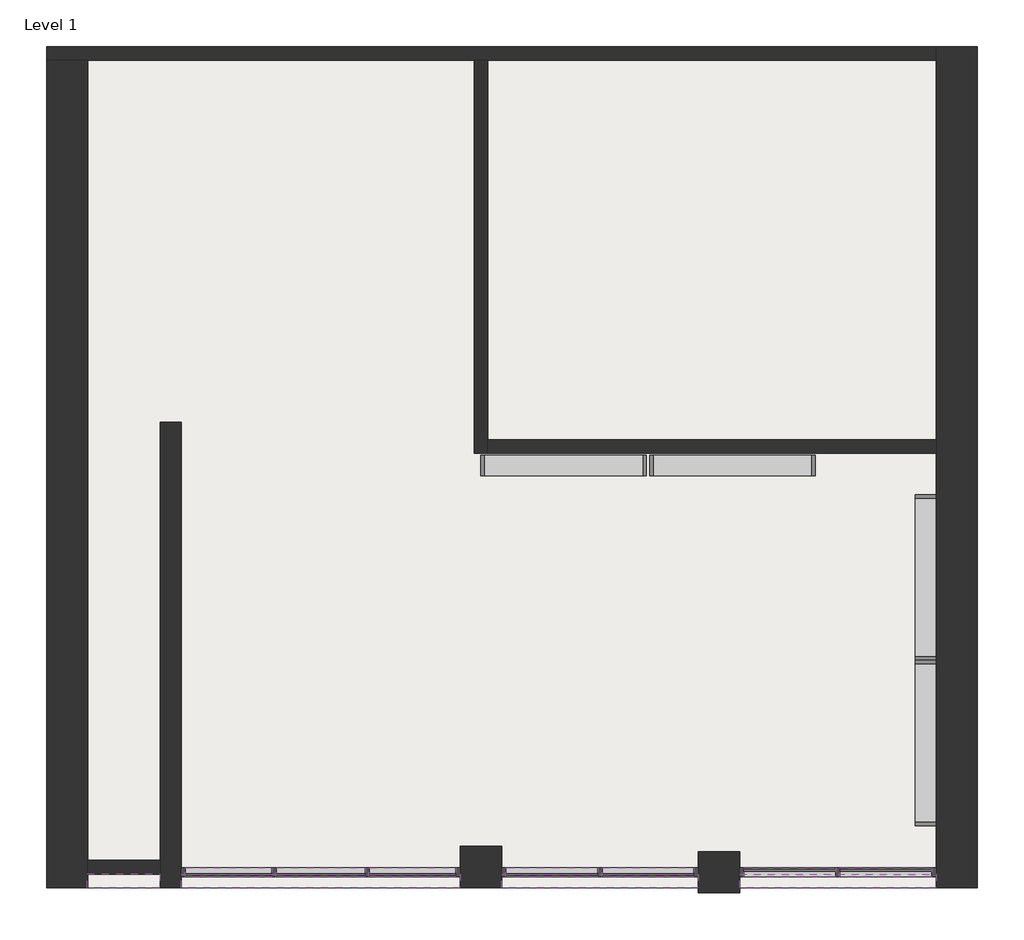
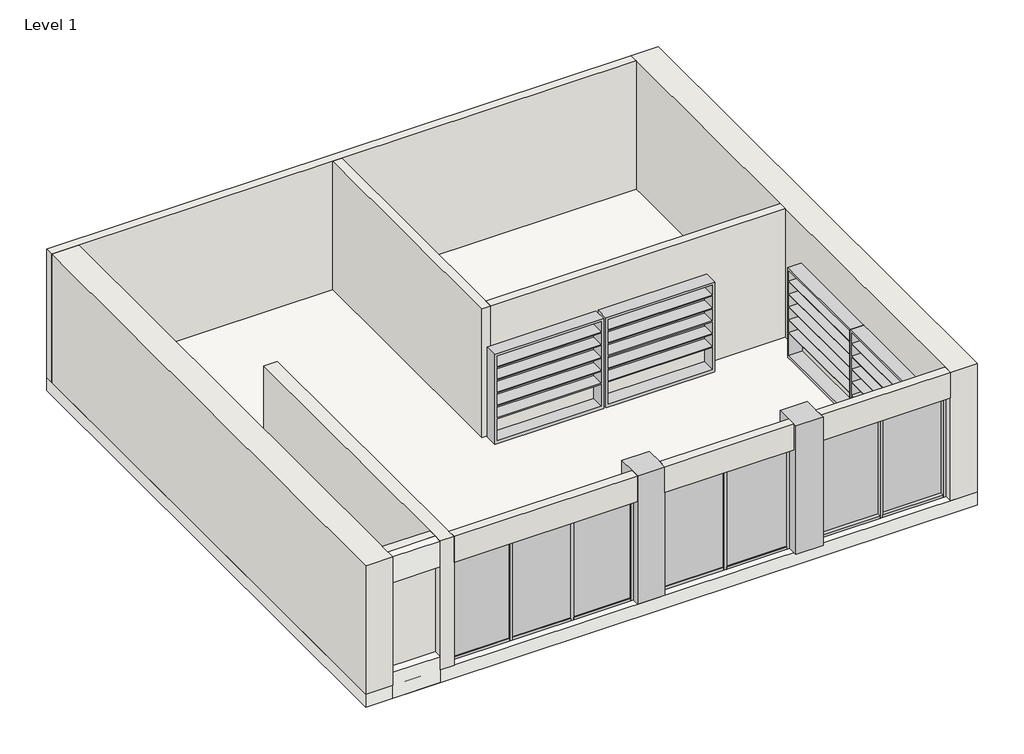
# One storey: 24 members, 10 walls, 7 plates, 4 furniture elements, 3 slabs, 2 columns.
"""IFC4 building model written with IfcOpenShell, lengths in millimetres."""

from ifc_helpers import new_model, si_unit, frame, origin, origin_with_axes, place, context, project, spatial, polyline, outline, extrude, faceted_brep, transform, mapped, element, save
from components import furniture_b1da5ad0, member_d37749d9, member_cba00588, member_20eb5ac3, member_f0fea5a5, member_ee409385, system_panel_glazed_612c9cdf, system_panel_glazed_17617b93, system_panel_glazed_febae1d4

model = new_model("IFC4")

# Units and contexts
model_context = context("Model", 3, world=origin())
ifc_project = project(units=[si_unit("LENGTHUNIT", "METRE", prefix="MILLI")], contexts=[model_context])

# Site, building, storey
site = spatial("IfcSite", under=ifc_project)
building = spatial("IfcBuilding", under=site)
storey = spatial("IfcBuildingStorey", under=building, Name="Level 1", Elevation=0.0)

# Columns
placement = place(None, origin())
element("IfcColumn", 1, ObjectType="Rectangular Column : 24\" x 24\" 2", at=placement, inside=storey, context=model_context, shape_type="Brep", body=[
    faceted_brep([(-12478.6104559, -292.271263, 0.0), (-12478.6104559, -901.871263, 0.0), (-13088.2104559, -901.871263, 0.0), (-13088.2104559, -292.271263, 0.0), (-12478.6104559, -292.271263, 3048.0), (-12478.6104559, -698.671263, 3048.0), (-12478.6104559, -901.871263, 3048.0), (-12478.6104559, -901.871263, 2438.4), (-13088.2104559, -901.871263, 3048.0), (-13088.2104559, -901.871263, 2438.4), (-13088.2104559, -698.671263, 3048.0), (-13088.2104559, -292.271263, 3048.0)], [[[0, 1, 2, 3]], [[4, 5, 6, 7, 1, 0]], [[6, 8, 9, 2, 1, 7]], [[8, 10, 11, 3, 2, 9]], [[11, 4, 0, 3]], [[4, 11, 10, 8, 6, 5]]]),
])
element("IfcColumn", 2, ObjectType="Rectangular Column : 24\" x 24\" 3", at=placement, inside=storey, context=model_context, shape_type="Brep", body=[
    faceted_brep([(-8973.4104559, -368.471263, 0.0), (-8973.4104559, -978.071263, 0.0), (-9583.0104559, -978.071263, 0.0), (-9583.0104559, -368.471263, 0.0), (-8973.4104559, -368.471263, 3048.0), (-8973.4104559, -698.671263, 3048.0), (-8973.4104559, -901.871263, 3048.0), (-8973.4104559, -978.071263, 3048.0), (-9583.0104559, -978.071263, 3048.0), (-9583.0104559, -901.871263, 3048.0), (-9583.0104559, -698.671263, 3048.0), (-9583.0104559, -368.471263, 3048.0)], [[[0, 1, 2, 3]], [[4, 5, 6, 7, 1, 0]], [[7, 8, 2, 1]], [[8, 9, 10, 11, 3, 2]], [[11, 4, 0, 3]], [[4, 11, 10, 9, 8, 7, 6, 5]]]),
])

# Furniture
furniture_shape = furniture_b1da5ad0(model_context)
element("IfcFurniture", 3, ObjectType="Shelving : 96\" x 12\" x 84\"", at=placement, inside=storey, context=model_context, shape_type="MappedRepresentation", body=[
    mapped(furniture_shape, transform((-11564.2104559, 5625.928737, 0.0), x_axis=(1.0, 0.0, 0.0), y_axis=(0.0, 1.0, 0.0), z_axis=(0.0, 0.0, 1.0))),
])
element("IfcFurniture", 4, ObjectType="Shelving : 96\" x 12\" x 84\"", at=placement, inside=storey, context=model_context, shape_type="MappedRepresentation", body=[
    mapped(furniture_shape, transform((-5925.4104559, 3670.128737, 0.0), x_axis=(0.0, -1.0, 0.0), y_axis=(1.0, 0.0, 0.0), z_axis=(0.0, 0.0, 1.0))),
])
element("IfcFurniture", 5, ObjectType="Shelving : 96\" x 12\" x 84\"", at=placement, inside=storey, context=model_context, shape_type="MappedRepresentation", body=[
    mapped(furniture_shape, transform((-9075.0104559, 5625.928737, 0.0), x_axis=(1.0, 0.0, 0.0), y_axis=(0.0, 1.0, 0.0), z_axis=(0.0, 0.0, 1.0))),
])
element("IfcFurniture", 6, ObjectType="Shelving : 96\" x 12\" x 84\"", at=placement, inside=storey, context=model_context, shape_type="MappedRepresentation", body=[
    mapped(furniture_shape, transform((-5927.4247367, 1231.728737, 0.0), x_axis=(0.0, -1.0, 0.0), y_axis=(1.0, 0.0, 0.0), z_axis=(0.0, 0.0, 1.0))),
])

# Members
member_shape = member_d37749d9(model_context)
element("IfcMember", 7, ObjectType="Rectangular Mullion : 2.5\" x 5\" rectangular", at=placement, inside=storey, context=model_context, shape_type="MappedRepresentation", body=[
    mapped(member_shape, transform((-14491.5604559, -673.271263, 0.0), x_axis=(0.0, 0.0, -1.0), y_axis=(0.0, 1.0, 0.0), z_axis=(1.0, 0.0, 0.0))),
])
member_2_shape = member_cba00588(model_context)
element("IfcMember", 8, ObjectType="Rectangular Mullion : 2.5\" x 5\" rectangular", at=placement, inside=storey, context=model_context, shape_type="MappedRepresentation", body=[
    mapped(member_2_shape, transform((-13151.7104559, -673.271263, 0.0), x_axis=(0.0, 0.0, -1.0), y_axis=(0.0, 1.0, 0.0), z_axis=(1.0, 0.0, 0.0))),
])
element("IfcMember", 9, ObjectType="Rectangular Mullion : 2.5\" x 5\" rectangular", at=placement, inside=storey, context=model_context, shape_type="MappedRepresentation", body=[
    mapped(member_2_shape, transform((-15863.1604559, -673.271263, 0.0), x_axis=(0.0, 0.0, -1.0), y_axis=(0.0, 1.0, 0.0), z_axis=(1.0, 0.0, 0.0))),
])
element("IfcMember", 10, ObjectType="Rectangular Mullion : 2.5\" x 5\" rectangular", at=placement, inside=storey, context=model_context, shape_type="MappedRepresentation", body=[
    mapped(member_2_shape, transform((-17139.5104559, -673.271263, 2438.4), x_axis=(0.0, 0.0, 1.0), y_axis=(0.0, 1.0, 0.0), z_axis=(-1.0, 0.0, 0.0))),
])
element("IfcMember", 11, ObjectType="Rectangular Mullion : 2.5\" x 5\" rectangular", at=placement, inside=storey, context=model_context, shape_type="MappedRepresentation", body=[
    mapped(member_2_shape, transform((-14428.0604559, -673.271263, 2438.4), x_axis=(0.0, 0.0, 1.0), y_axis=(0.0, 1.0, 0.0), z_axis=(-1.0, 0.0, 0.0))),
])
element("IfcMember", 12, ObjectType="Rectangular Mullion : 2.5\" x 5\" rectangular", at=placement, inside=storey, context=model_context, shape_type="MappedRepresentation", body=[
    mapped(member_shape, transform((-15799.6604559, -673.271263, 2438.4), x_axis=(0.0, 0.0, 1.0), y_axis=(0.0, 1.0, 0.0), z_axis=(-1.0, 0.0, 0.0))),
])
member_3_shape = member_20eb5ac3(model_context)
element("IfcMember", 13, ObjectType="Rectangular Mullion : 2.5\" x 5\" rectangular", at=placement, inside=storey, context=model_context, shape_type="MappedRepresentation", body=[
    mapped(member_3_shape, transform((-12415.1104559, -673.271263, 2438.4), x_axis=(0.0, 0.0, 1.0), y_axis=(0.0, 1.0, 0.0), z_axis=(-1.0, 0.0, 0.0))),
])
element("IfcMember", 14, ObjectType="Rectangular Mullion : 2.5\" x 5\" rectangular", at=placement, inside=storey, context=model_context, shape_type="MappedRepresentation", body=[
    mapped(member_3_shape, transform((-6141.3104559, -673.271263, 2438.4), x_axis=(0.0, 0.0, 1.0), y_axis=(0.0, -1.0, 0.0), z_axis=(1.0, 0.0, 0.0))),
])
element("IfcMember", 15, ObjectType="Rectangular Mullion : 2.5\" x 5\" rectangular", at=placement, inside=storey, context=model_context, shape_type="MappedRepresentation", body=[
    mapped(member_3_shape, transform((-10999.0604559, -673.271263, 2438.4), x_axis=(0.0, 0.0, 1.0), y_axis=(0.0, 1.0, 0.0), z_axis=(-1.0, 0.0, 0.0))),
])
element("IfcMember", 16, ObjectType="Rectangular Mullion : 2.5\" x 5\" rectangular", at=placement, inside=storey, context=model_context, shape_type="MappedRepresentation", body=[
    mapped(member_3_shape, transform((-7557.3604559, -673.271263, 2438.4), x_axis=(0.0, 0.0, 1.0), y_axis=(0.0, -1.0, 0.0), z_axis=(1.0, 0.0, 0.0))),
])
element("IfcMember", 17, ObjectType="Rectangular Mullion : 2.5\" x 5\" rectangular", at=placement, inside=storey, context=model_context, shape_type="MappedRepresentation", body=[
    mapped(member_3_shape, transform((-9646.5104559, -673.271263, 0.0), x_axis=(0.0, 0.0, -1.0), y_axis=(0.0, 1.0, 0.0), z_axis=(1.0, 0.0, 0.0))),
])
element("IfcMember", 18, ObjectType="Rectangular Mullion : 2.5\" x 5\" rectangular", at=placement, inside=storey, context=model_context, shape_type="MappedRepresentation", body=[
    mapped(member_3_shape, transform((-8909.9104559, -673.271263, 0.0), x_axis=(0.0, 0.0, -1.0), y_axis=(0.0, -1.0, 0.0), z_axis=(-1.0, 0.0, 0.0))),
])
element("IfcMember", 19, ObjectType="Rectangular Mullion : 2.5\" x 5\" rectangular", at=placement, inside=storey, context=model_context, shape_type="MappedRepresentation", body=[
    mapped(member_3_shape, transform((-11062.5604559, -673.271263, 0.0), x_axis=(0.0, 0.0, -1.0), y_axis=(0.0, 1.0, 0.0), z_axis=(1.0, 0.0, 0.0))),
])
element("IfcMember", 20, ObjectType="Rectangular Mullion : 2.5\" x 5\" rectangular", at=placement, inside=storey, context=model_context, shape_type="MappedRepresentation", body=[
    mapped(member_3_shape, transform((-7493.8604559, -673.271263, 0.0), x_axis=(0.0, 0.0, -1.0), y_axis=(0.0, -1.0, 0.0), z_axis=(-1.0, 0.0, 0.0))),
])
member_4_shape = member_f0fea5a5(model_context)
element("IfcMember", 21, ObjectType="Rectangular Mullion : 2.5\" x 5\" rectangular", at=placement, inside=storey, context=model_context, shape_type="MappedRepresentation", body=[
    mapped(member_4_shape, transform((-14459.8104559, -673.271263, 0.0), x_axis=(-1.0, 0.0, 0.0), y_axis=(0.0, 1.0, 0.0), z_axis=(0.0, 0.0, -1.0))),
])
element("IfcMember", 22, ObjectType="Rectangular Mullion : 2.5\" x 5\" rectangular", at=placement, inside=storey, context=model_context, shape_type="MappedRepresentation", body=[
    mapped(member_4_shape, transform((-15831.4104559, -673.271263, 0.0), x_axis=(-1.0, 0.0, 0.0), y_axis=(0.0, 1.0, 0.0), z_axis=(0.0, 0.0, -1.0))),
])
element("IfcMember", 23, ObjectType="Rectangular Mullion : 2.5\" x 5\" rectangular", at=placement, inside=storey, context=model_context, shape_type="MappedRepresentation", body=[
    mapped(member_4_shape, transform((-11030.8104559, -673.271263, 0.0), x_axis=(-1.0, 0.0, 0.0), y_axis=(0.0, 1.0, 0.0), z_axis=(0.0, 0.0, -1.0))),
])
element("IfcMember", 24, ObjectType="Rectangular Mullion : 2.5\" x 5\" rectangular", at=placement, inside=storey, context=model_context, shape_type="MappedRepresentation", body=[
    mapped(member_4_shape, transform((-7525.6104559, -673.271263, 0.0), x_axis=(1.0, 0.0, 0.0), y_axis=(0.0, -1.0, 0.0), z_axis=(0.0, 0.0, -1.0))),
])
member_5_shape = member_ee409385(model_context)
element("IfcMember", 25, ObjectType="Rectangular Mullion : 2.5\" x 5\" rectangular", at=placement, inside=storey, context=model_context, shape_type="MappedRepresentation", body=[
    mapped(member_5_shape, transform((-17203.0104559, -673.271263, 0.0), x_axis=(-1.0, 0.0, 0.0), y_axis=(0.0, 1.0, 0.0), z_axis=(0.0, 0.0, -1.0))),
])
element("IfcMember", 26, ObjectType="Rectangular Mullion : 2.5\" x 5\" rectangular", at=placement, inside=storey, context=model_context, shape_type="MappedRepresentation", body=[
    mapped(member_5_shape, transform((-12478.6104559, -673.271263, 0.0), x_axis=(-1.0, 0.0, 0.0), y_axis=(0.0, 1.0, 0.0), z_axis=(0.0, 0.0, -1.0))),
])
element("IfcMember", 27, ObjectType="Rectangular Mullion : 2.5\" x 5\" rectangular", at=placement, inside=storey, context=model_context, shape_type="MappedRepresentation", body=[
    mapped(member_5_shape, transform((-6077.8104559, -673.271263, 0.0), x_axis=(1.0, 0.0, 0.0), y_axis=(0.0, -1.0, 0.0), z_axis=(0.0, 0.0, -1.0))),
])
element("IfcMember", 28, ObjectType="Rectangular Mullion : 2.5\" x 5\" rectangular", at=placement, inside=storey, context=model_context, shape_type="MappedRepresentation", body=[
    mapped(member_5_shape, transform((-13088.2104559, -673.271263, 2438.4), x_axis=(1.0, 0.0, 0.0), y_axis=(0.0, 1.0, 0.0), z_axis=(0.0, 0.0, 1.0))),
])
element("IfcMember", 29, ObjectType="Rectangular Mullion : 2.5\" x 5\" rectangular", at=placement, inside=storey, context=model_context, shape_type="MappedRepresentation", body=[
    mapped(member_5_shape, transform((-9583.0104559, -673.271263, 2438.4), x_axis=(1.0, 0.0, 0.0), y_axis=(0.0, 1.0, 0.0), z_axis=(0.0, 0.0, 1.0))),
])
element("IfcMember", 30, ObjectType="Rectangular Mullion : 2.5\" x 5\" rectangular", at=placement, inside=storey, context=model_context, shape_type="MappedRepresentation", body=[
    mapped(member_5_shape, transform((-8973.4104559, -673.271263, 2438.4), x_axis=(-1.0, 0.0, 0.0), y_axis=(0.0, -1.0, 0.0), z_axis=(0.0, 0.0, 1.0))),
])

# Plates
system_panel_glazed_shape = system_panel_glazed_612c9cdf(model_context)
element("IfcPlate", 31, ObjectType="System Panel : Glazed", at=placement, inside=storey, context=model_context, shape_type="MappedRepresentation", body=[
    mapped(system_panel_glazed_shape, transform((-13789.8854559, -673.271263, 63.5), x_axis=(-1.0, 0.0, 0.0), y_axis=(0.0, -1.0, 0.0), z_axis=(0.0, 0.0, 1.0))),
])
element("IfcPlate", 32, ObjectType="System Panel : Glazed", at=placement, inside=storey, context=model_context, shape_type="MappedRepresentation", body=[
    mapped(system_panel_glazed_shape, transform((-16501.3354559, -673.271263, 63.5), x_axis=(-1.0, 0.0, 0.0), y_axis=(0.0, -1.0, 0.0), z_axis=(0.0, 0.0, 1.0))),
])
system_panel_glazed_2_shape = system_panel_glazed_17617b93(model_context)
element("IfcPlate", 33, ObjectType="System Panel : Glazed", at=placement, inside=storey, context=model_context, shape_type="MappedRepresentation", body=[
    mapped(system_panel_glazed_2_shape, transform((-15145.6104559, -673.271263, 63.5), x_axis=(-1.0, 0.0, 0.0), y_axis=(0.0, -1.0, 0.0), z_axis=(0.0, 0.0, 1.0))),
])
system_panel_glazed_3_shape = system_panel_glazed_febae1d4(model_context)
element("IfcPlate", 34, ObjectType="System Panel : Glazed", at=placement, inside=storey, context=model_context, shape_type="MappedRepresentation", body=[
    mapped(system_panel_glazed_3_shape, transform((-10322.7854559, -673.271263, 63.5), x_axis=(-1.0, 0.0, 0.0), y_axis=(0.0, -1.0, 0.0), z_axis=(0.0, 0.0, 1.0))),
])
element("IfcPlate", 35, ObjectType="System Panel : Glazed", at=placement, inside=storey, context=model_context, shape_type="MappedRepresentation", body=[
    mapped(system_panel_glazed_3_shape, transform((-8233.6354559, -673.271263, 63.5), x_axis=(1.0, 0.0, 0.0), y_axis=(0.0, 1.0, 0.0), z_axis=(0.0, 0.0, 1.0))),
])
element("IfcPlate", 36, ObjectType="System Panel : Glazed", at=placement, inside=storey, context=model_context, shape_type="MappedRepresentation", body=[
    mapped(system_panel_glazed_3_shape, transform((-11738.8354559, -673.271263, 63.5), x_axis=(-1.0, 0.0, 0.0), y_axis=(0.0, -1.0, 0.0), z_axis=(0.0, 0.0, 1.0))),
])
element("IfcPlate", 37, ObjectType="System Panel : Glazed", at=placement, inside=storey, context=model_context, shape_type="MappedRepresentation", body=[
    mapped(system_panel_glazed_3_shape, transform((-6817.5854559, -673.271263, 63.5), x_axis=(1.0, 0.0, 0.0), y_axis=(0.0, 1.0, 0.0), z_axis=(0.0, 0.0, 1.0))),
])

# Slabs
element("IfcSlab", 38, ObjectType="wall design", at=placement, inside=storey, context=model_context, shape_type="SweptSolid", body=[
    extrude(outline(polyline([(-17507.8104559, -698.671263), (-17507.8104559, -901.871263), (-18574.6104559, -901.871263), (-18574.6104559, -698.671263), (-17507.8104559, -698.671263)])), frame((0.0, 0.0, -304.8), z_axis=(0.0, 0.0, 1.0), x_axis=(1.0, 0.0, 0.0)), (0.0, 0.0, 1.0), 609.6),
])
element("IfcSlab", 39, ObjectType="wall design", at=placement, inside=storey, context=model_context, shape_type="SweptSolid", body=[
    extrude(outline(polyline([(-17519.2074726, -697.3682798), (-17519.2074726, -900.5682798), (-18586.0074726, -900.5682798), (-18586.0074726, -697.3682798), (-17519.2074726, -697.3682798)])), frame((0.0, 0.0, 2438.4), z_axis=(0.0, 0.0, 1.0), x_axis=(1.0, 0.0, 0.0)), (0.0, 0.0, 1.0), 609.6),
])
element("IfcSlab", 40, ObjectType="white floor", at=placement, inside=storey, context=model_context, shape_type="SweptSolid", body=[
    extrude(outline(polyline([(-5468.2104559, 11493.328737), (-5468.2104559, -901.871263), (-19184.2104559, -901.871263), (-19184.2104559, 11493.328737), (-5468.2104559, 11493.328737)])), frame((0.0, 0.0, -304.8), z_axis=(0.0, 0.0, 1.0), x_axis=(1.0, 0.0, 0.0)), (0.0, 0.0, 1.0), 304.8),
])

# Walls
element("IfcWall", 41, ObjectType="Generic - 12\" 2", at=placement, inside=storey, context=model_context, shape_type="Brep", body=[
    faceted_brep([(-17203.0104559, -901.871263, 0.0), (-17203.0104559, 5956.128737, 0.0), (-17203.0104559, 5956.128737, 3048.0), (-17203.0104559, -698.671263, 3048.0), (-17203.0104559, -901.871263, 3048.0), (-17203.0104559, -901.871263, 2438.4), (-17507.8104559, -901.871263, 0.0), (-17507.8104559, -901.871263, 3048.0), (-17507.8104559, -698.671263, 3048.0), (-17507.8104559, -495.471263, 3048.0), (-17507.8104559, 5956.128737, 3048.0), (-17507.8104559, 5956.128737, 0.0), (-17507.8104559, -495.471263, 0.0), (-17507.8104559, -698.671263, 0.0)], [[[0, 1, 2, 3, 4, 5]], [[6, 7, 8, 9, 10, 11, 12, 13]], [[1, 0, 6, 13, 12, 11]], [[2, 1, 11, 10]], [[0, 5, 4, 7, 6]], [[4, 3, 2, 10, 9, 8, 7]]]),
])
element("IfcWall", 42, ObjectType="Generic - 2'", at=placement, inside=storey, context=model_context, shape_type="Brep", body=[
    faceted_brep([(-18574.6104559, -901.871263, 0.0), (-18574.6104559, -698.671263, 0.0), (-18574.6104559, -495.471263, 0.0), (-18574.6104559, 11290.128737, 0.0), (-18574.6104559, 11290.128737, 3048.0), (-18574.6104559, -495.471263, 3048.0), (-18574.6104559, -698.671263, 3048.0), (-18574.6104559, -901.871263, 3048.0), (-19184.2104559, -901.871263, 0.0), (-19184.2104559, -901.871263, 3048.0), (-19184.2104559, 11290.128737, 3048.0), (-19184.2104559, 11290.128737, 0.0)], [[[0, 1, 2, 3, 4, 5, 6, 7]], [[8, 9, 10, 11]], [[3, 2, 1, 0, 8, 11]], [[0, 7, 9, 8]], [[4, 3, 11, 10]], [[7, 6, 5, 4, 10, 9]]]),
])
element("IfcWall", 43, ObjectType="Generic - 2'", at=placement, inside=storey, context=model_context, shape_type="Brep", body=[
    faceted_brep([(-6077.8104559, 11493.328737, 0.0), (-6077.8104559, 11290.128737, 0.0), (-6077.8104559, 5702.128737, 0.0), (-6077.8104559, 5498.928737, 0.0), (-6077.8104559, -901.871263, 0.0), (-6077.8104559, -901.871263, 2438.4), (-6077.8104559, -901.871263, 3048.0), (-6077.8104559, -698.671263, 3048.0), (-6077.8104559, 5498.928737, 3048.0), (-6077.8104559, 5702.128737, 3048.0), (-6077.8104559, 11290.128737, 3048.0), (-6077.8104559, 11493.328737, 3048.0), (-5468.2104559, 11493.328737, 0.0), (-5468.2104559, 11493.328737, 3048.0), (-5468.2104559, -901.871263, 3048.0), (-5468.2104559, -901.871263, 0.0)], [[[0, 1, 2, 3, 4, 5, 6, 7, 8, 9, 10, 11]], [[12, 13, 14, 15]], [[4, 3, 2, 1, 0, 12, 15]], [[0, 11, 13, 12]], [[6, 5, 4, 15, 14]], [[11, 10, 9, 8, 7, 6, 14, 13]]]),
])
element("IfcWall", 44, ObjectType="Generic - 8\"", at=placement, inside=storey, context=model_context, shape_type="SweptSolid", body=[
    extrude(outline(polyline([(-17203.0104559, -698.671263), (-13088.2104559, -698.671263), (-13088.2104559, -901.871263), (-17203.0104559, -901.871263), (-17203.0104559, -698.671263)])), frame((0.0, 0.0, 2438.4), z_axis=(0.0, 0.0, 1.0), x_axis=(1.0, 0.0, 0.0)), (0.0, 0.0, 1.0), 609.6),
])
element("IfcWall", 45, ObjectType="Generic - 8\"", at=placement, inside=storey, context=model_context, shape_type="SweptSolid", body=[
    extrude(outline(polyline([(-12478.6104559, -698.671263), (-9583.0104559, -698.671263), (-9583.0104559, -901.871263), (-12478.6104559, -901.871263), (-12478.6104559, -698.671263)])), frame((0.0, 0.0, 2438.4), z_axis=(0.0, 0.0, 1.0), x_axis=(1.0, 0.0, 0.0)), (0.0, 0.0, 1.0), 609.6),
])
element("IfcWall", 46, ObjectType="Generic - 8\"", at=placement, inside=storey, context=model_context, shape_type="SweptSolid", body=[
    extrude(outline(polyline([(-8973.4104559, -698.671263), (-6077.8104559, -698.671263), (-6077.8104559, -901.871263), (-8973.4104559, -901.871263), (-8973.4104559, -698.671263)])), frame((0.0, 0.0, 2438.4), z_axis=(0.0, 0.0, 1.0), x_axis=(1.0, 0.0, 0.0)), (0.0, 0.0, 1.0), 609.6),
])
element("IfcWall", 47, ObjectType="Generic - 8\" 2", at=placement, inside=storey, context=model_context, shape_type="Brep", body=[
    faceted_brep([(-19184.2104559, 11290.128737, 0.0), (-18574.6104559, 11290.128737, 0.0), (-12885.0104559, 11290.128737, 0.0), (-12681.8104559, 11290.128737, 0.0), (-6077.8104559, 11290.128737, 0.0), (-6077.8104559, 11290.128737, 3048.0), (-12681.8104559, 11290.128737, 3048.0), (-12885.0104559, 11290.128737, 3048.0), (-18574.6104559, 11290.128737, 3048.0), (-19184.2104559, 11290.128737, 3048.0), (-19184.2104559, 11493.328737, 0.0), (-19184.2104559, 11493.328737, 3048.0), (-6077.8104559, 11493.328737, 3048.0), (-6077.8104559, 11493.328737, 0.0)], [[[0, 1, 2, 3, 4, 5, 6, 7, 8, 9]], [[10, 11, 12, 13]], [[4, 3, 2, 1, 0, 10, 13]], [[0, 9, 11, 10]], [[5, 4, 13, 12]], [[9, 8, 7, 6, 5, 12, 11]]]),
])
element("IfcWall", 48, ObjectType="Generic - 8\" 2", at=placement, inside=storey, context=model_context, shape_type="Brep", body=[
    faceted_brep([(-12885.0104559, 11290.128737, 0.0), (-12885.0104559, 5498.928737, 0.0), (-12885.0104559, 5498.928737, 3048.0), (-12885.0104559, 11290.128737, 3048.0), (-12681.8104559, 11290.128737, 0.0), (-12681.8104559, 11290.128737, 3048.0), (-12681.8104559, 5702.128737, 3048.0), (-12681.8104559, 5498.928737, 3048.0), (-12681.8104559, 5498.928737, 0.0), (-12681.8104559, 5702.128737, 0.0)], [[[0, 1, 2, 3]], [[4, 5, 6, 7, 8, 9]], [[1, 0, 4, 9, 8]], [[0, 3, 5, 4]], [[2, 1, 8, 7]], [[3, 2, 7, 6, 5]]]),
])
element("IfcWall", 49, ObjectType="Generic - 8\" 2", at=placement, inside=storey, context=model_context, shape_type="SweptSolid", body=[
    extrude(outline(polyline([(-6077.8104559, 5498.928737), (-12681.8104559, 5498.928737), (-12681.8104559, 5702.128737), (-6077.8104559, 5702.128737), (-6077.8104559, 5498.928737)])), origin_with_axes(), (0.0, 0.0, 1.0), 3048.0),
])
element("IfcWall", 50, ObjectType="Generic - 8\" 2", at=placement, inside=storey, context=model_context, shape_type="SweptSolid", body=[
    extrude(outline(polyline([(-17507.8104559, -698.671263), (-18574.6104559, -698.671263), (-18574.6104559, -495.471263), (-17507.8104559, -495.471263), (-17507.8104559, -698.671263)])), origin_with_axes(), (0.0, 0.0, 1.0), 3048.0),
])

save(model, "model.ifc")

# Revit data of these elements
# Type "Rectangular Column : 24\" x 24\" 2"
#   Assembly Code = "B1010200"
#   Depth = 2' - 0"
#   Offset Base = 0' - 0"
#   Offset Top = 0' - 0"
#   Width = 2' - 0"
#   Material = Parking Stripe
# Type "Rectangular Column : 24\" x 24\" 3"
#   Assembly Code = "B1010200"
#   Depth = 2' - 0"
#   Offset Base = 0' - 0"
#   Offset Top = 0' - 0"
#   Width = 2' - 0"
#   Material = Roofing, EPDM Membrane
# Type "Shelving : 96\" x 12\" x 84\""
#   Assembly Code = "E2020200"
#   Depth = 1' - 0"
#   Height = 7' - 0"
#   Width = 8' - 0"
#   Shelving Unit Material = Laminate, Ivory, Matte
#   Default Elevation = 0
# Type "Rectangular Mullion : 2.5\" x 5\" rectangular"
#   built-in parameter 1007304 = 0.416667 (stored number, unit not read)
#   built-in parameter 1007301 = 0.104167 (stored number, unit not read)
#   built-in parameter 1007300 = 0.104167 (stored number, unit not read)
# Type "System Panel : Glazed"
#   Construction Type Id = "GSP4R"
#   Analytic Construction = "1/8 in Pilkington single glazing"
#   Visual Light Transmittance = 0.9
#   Solar Heat Gain Coefficient = 0.86
#   Heat Transfer Coefficient (U) = 1.18115 BTU/(h·ft²·°F)
# Type "wall design"
#   Assembly Code = "B1010"
#   Function = 0
#   Layers, outside or top first: 2' - 0" "Damp-proofing" (function 1)
# Type "white floor"
#   Assembly Code = "B1010"
#   Function = 0
#   Layers, outside or top first: 1' - 0" "Gypsum Wall Board" (function 1)
# Type "Generic - 12\" 2"
#   Assembly Code = "B2010"
#   Layers, outside or top first: 1' - 0" "Parking Stripe" (function 1)
# Type "Generic - 2'"
#   Assembly Code = "B2010"
#   Layers, outside or top first: 2' - 0" "Acoustic Ceiling Tile 24 x 24" (function 1)
# Type "Generic - 8\""
#   Assembly Code = "B2010"
#   Layers, outside or top first: 0' - 8" "Roofing, EPDM Membrane" (function 1)
# Type "Generic - 8\" 2"
#   Assembly Code = "B2010"
#   Layers, outside or top first: 0' - 8" "Parking Stripe" (function 1)
# Element 1 (IfcColumn, "Rectangular Column : 24\" x 24\" 2")
#   Phase Created = New Construction
#   Materials on its faces: "Parking Stripe"
# Element 2 (IfcColumn, "Rectangular Column : 24\" x 24\" 3")
#   Phase Created = New Construction
#   Materials on its faces: "Roofing, EPDM Membrane"
# Elements 3, 4, 5, 6 (IfcFurniture, "Shelving : 96\" x 12\" x 84\"")
#   Phase Created = New Construction
#   Materials on its faces: "Laminate, Ivory, Matte"
# Elements 7, 8, 9, 10, 11, 12, 13, 14, 15, 16, 17, 18, 19, 20, 21, 22, 23, 24, 25, 26, 27, 28, 29, 30 (IfcMember, "Rectangular Mullion : 2.5\" x 5\" rectangular")
#   Phase Created = New Construction
#   Materials on its faces: "Iron, Ductile"
# Elements 31, 32, 33, 34, 35, 36, 37 (IfcPlate, "System Panel : Glazed")
#   Phase Created = New Construction
#   Materials on its faces: "Glass"
# Element 38 (IfcSlab, "wall design")
#   Height Offset From Level = 1' - 0"
#   Phase Created = New Construction
#   Materials on its faces: "Damp-proofing"
# Element 39 (IfcSlab, "wall design")
#   Height Offset From Level = 10' - 0"
#   Phase Created = New Construction
#   Materials on its faces: "Damp-proofing"
# Element 40 (IfcSlab, "white floor")
#   Height Offset From Level = 0' - 0"
#   Phase Created = New Construction
#   Materials on its faces: "Gypsum Wall Board"
# Element 41 (IfcWall, "Generic - 12\" 2")
#   Top Offset = 0' - 0"
#   Base Offset = 0' - 0"
#   Unconnected Height = 10' - 0"
#   wall height = 10' - 0"
#   Phase Created = New Construction
#   Base Constraint = Level 1
#   Materials on its faces: "Parking Stripe", "Acoustic Ceiling Tile 24 x 24"
# Element 42 (IfcWall, "Generic - 2'")
#   Top Offset = 0' - 0"
#   Base Offset = 0' - 0"
#   Unconnected Height = 10' - 0"
#   wall height = 10' - 0"
#   Phase Created = New Construction
#   Base Constraint = Level 1
#   Materials on its faces: "Acoustic Ceiling Tile 24 x 24"
# Element 43 (IfcWall, "Generic - 2'")
#   Top Offset = 0' - 0"
#   Base Offset = 0' - 0"
#   Unconnected Height = 10' - 0"
#   wall height = 10' - 0"
#   Phase Created = New Construction
#   Base Constraint = Level 1
#   Materials on its faces: "Acoustic Ceiling Tile 24 x 24", "Parking Stripe"
# Elements 44, 45, 46 (IfcWall, "Generic - 8\"")
#   built-in parameter 1001111 = 8' - 0"
#   Top Offset = 0' - 0"
#   Base Offset = 8' - 0"
#   Unconnected Height = 2' - 0"
#   wall height = 2' - 0"
#   Phase Created = New Construction
#   Base Constraint = Level 1
#   Materials on its faces: "Roofing, EPDM Membrane"
# Element 47 (IfcWall, "Generic - 8\" 2")
#   Top Offset = 0' - 0"
#   Base Offset = 0' - 0"
#   Unconnected Height = 10' - 0"
#   wall height = 10' - 0"
#   Phase Created = New Construction
#   Base Constraint = Level 1
#   Materials on its faces: "Parking Stripe", "Acoustic Ceiling Tile 24 x 24"
# Elements 48, 49, 50 (IfcWall, "Generic - 8\" 2")
#   Top Offset = 0' - 0"
#   Base Offset = 0' - 0"
#   Unconnected Height = 10' - 0"
#   wall height = 10' - 0"
#   Phase Created = New Construction
#   Base Constraint = Level 1
#   Materials on its faces: "Parking Stripe"
# Materials
#   "Parking Stripe": class "Paint", colour RGB 250 250 91, transparency 0, Cost = 0
#   "Roofing, EPDM Membrane": class "Generic", colour RGB 127 127 127, transparency 0, Description = "EPDM roof membrane", Cost = 0
#   "Laminate, Ivory, Matte": class "Plastic", colour RGB 247 247 239, transparency 0, Description = "Plastic Laminate - Ivory, Matte", Cost = 0
#   "Damp-proofing": class "Generic", colour RGB 127 127 127, transparency 0, Description = "Damp-proofing", Cost = 0
#   "Gypsum Wall Board": class "Generic", colour RGB 127 127 127, transparency 0, Description = "Gypsum Wall Board", Cost = 0
#   "Acoustic Ceiling Tile 24 x 24": class "Generic", colour RGB 232 232 232, transparency 0, Description = "Acoustic Ceiling Tile 24 x 24", Cost = 0
#   "Iron, Ductile": class "Metal", colour RGB 0 0 0, transparency 0, Description = "Ductile cast iron", Cost = 0
#   "Glass": class "Glass", colour RGB 0 128 192, transparency 0.75, Description = "Soda Lime Glass", Cost = 0
